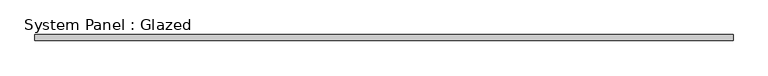
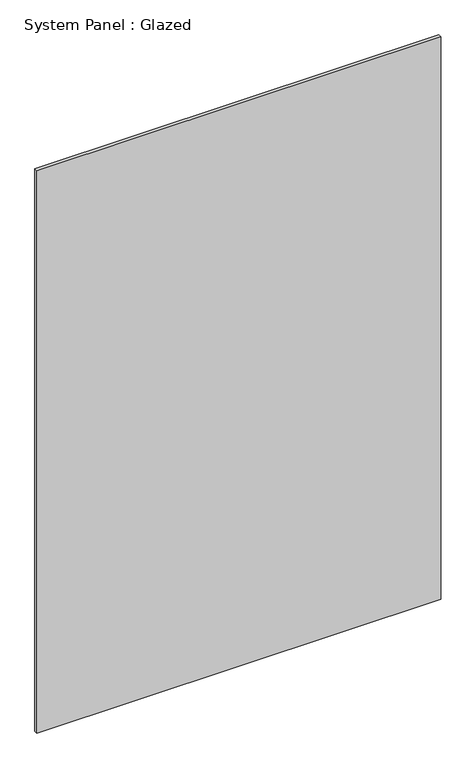
"""IFC4 building model written with IfcOpenShell, lengths in millimetres: plate geometry, System Panel : Glazed."""

from ifc_helpers import new_model, si_unit, origin, origin_with_axes, place, context, project, spatial, polyline, outline, extrude, source, transform, mapped, element, save


def system_panel_glazed_1f819173(model_context):
    return source(origin(), model_context, "Body", "SweptSolid", [
        extrude(outline(polyline([(1460.5, 19.05), (-1460.5, 19.05), (-1460.5, 44.45), (1460.5, 44.45), (1460.5, 19.05)])), origin_with_axes(), (0.0, 0.0, 1.0), 4301.3049749),
    ])


if __name__ == "__main__":
    model = new_model("IFC4")
    model_context = context("Model", 3, world=origin())
    ifc_project = project(units=[si_unit("LENGTHUNIT", "METRE", prefix="MILLI")], contexts=[model_context])
    site = spatial("IfcSite", under=ifc_project)
    building = spatial("IfcBuilding", under=site)
    placement = place(None, origin())
    system_panel_glazed_shape = system_panel_glazed_1f819173(model_context)
    element("IfcPlate", 1, ObjectType="System Panel : Glazed", at=placement, inside=building, context=model_context, shape_type="MappedRepresentation", body=[
        mapped(system_panel_glazed_shape, transform((0.0, 0.0, 0.0), x_axis=(1.0, 0.0, 0.0), y_axis=(0.0, 1.0, 0.0), z_axis=(0.0, 0.0, 1.0))),
    ])
    save(model, "model.ifc")

# Revit data of these elements
# Type "System Panel : Glazed"
#   Construction Type Id = "GSP4R"
#   Analytic Construction = "1/8 in Pilkington single glazing"
#   Visual Light Transmittance = 0.9
#   Solar Heat Gain Coefficient = 0.86
#   Heat Transfer Coefficient (U) = 1.18115 BTU/(h·ft²·°F)
# Element 1 (IfcPlate, "System Panel : Glazed")
#   Materials on its faces: "Glass"
# Materials
#   "Glass": class "Glass", colour RGB 0 128 192, transparency 0.75, Description = "Soda Lime Glass", Cost = 0
